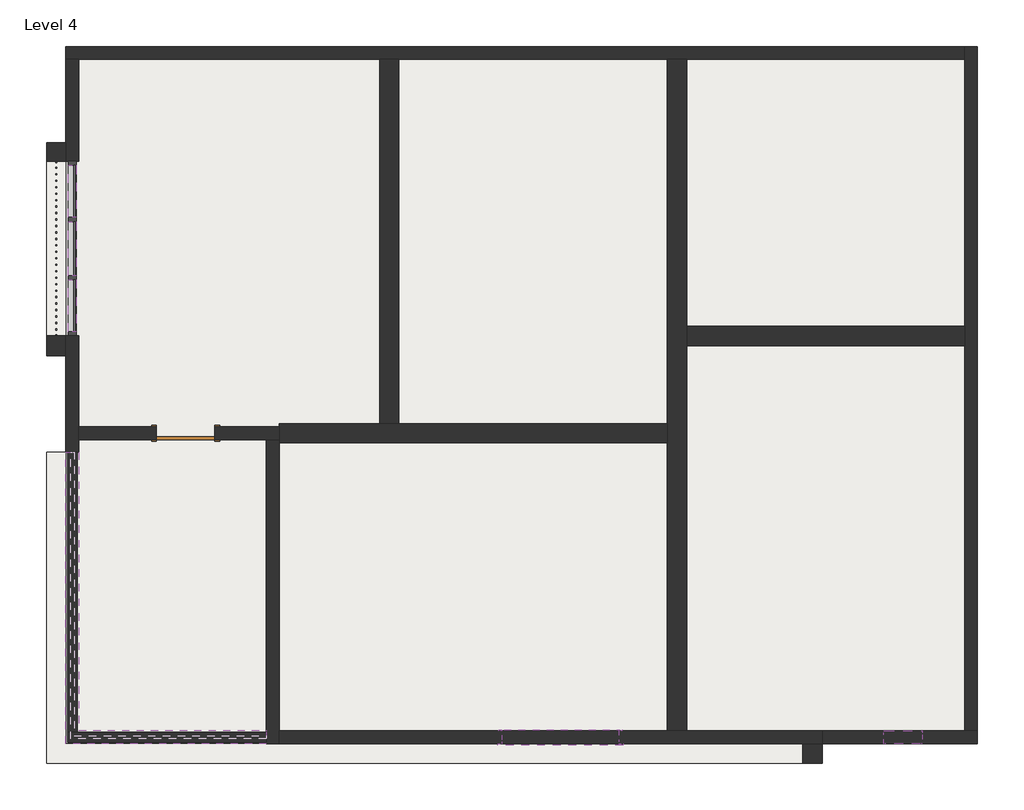
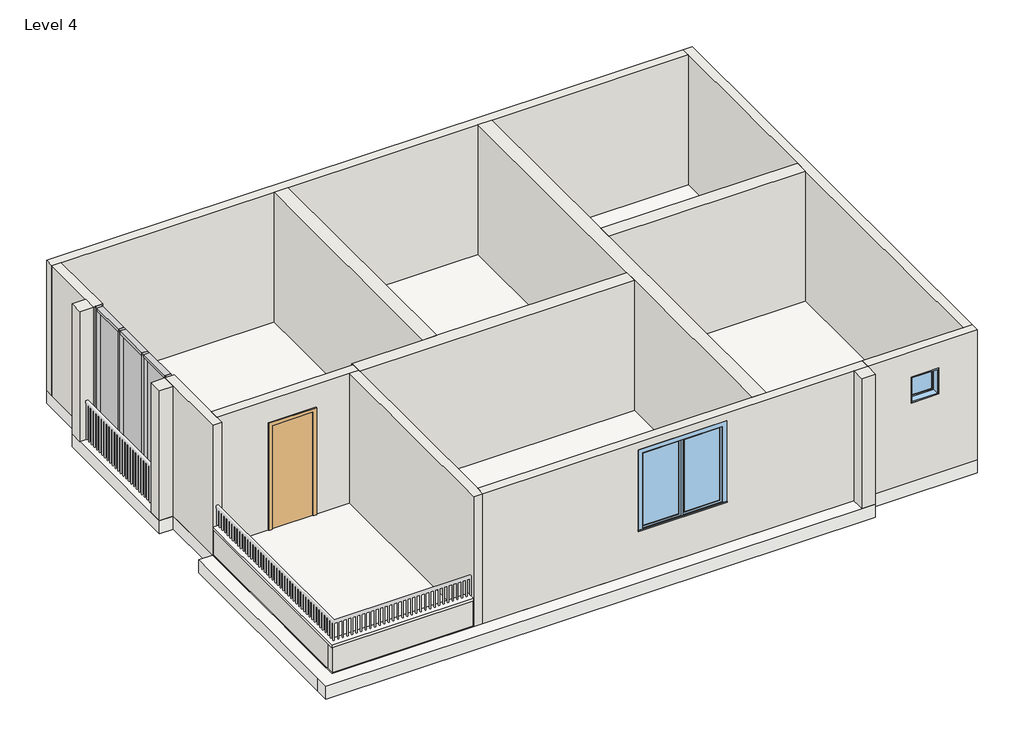
# One storey, part 1 of 2: 17 walls, 10 members, 3 plates, 3 slabs, 2 windows, 1 door.
"""IFC4 building model written with IfcOpenShell, lengths in millimetres."""

from ifc_helpers import new_model, si_unit, frame, origin, place, context, project, spatial, polyline, outline, extrude, faceted_brep, transform, mapped, element, save
from components import door_f936a269, member_eaba9652, member_3f395ae9, member_c17f1be2, member_d2e7e466, system_panel_glazed_52d31088, system_panel_glazed_f0722de2, window_97c6202a, window_6846e476

model = new_model("IFC4")

# Units and contexts
model_context = context("Model", 3, world=origin())
ifc_project = project(units=[si_unit("LENGTHUNIT", "METRE", prefix="MILLI")], contexts=[model_context])

# Site, building, storey
site = spatial("IfcSite", under=ifc_project)
building = spatial("IfcBuilding", under=site)
storey = spatial("IfcBuildingStorey", under=building, Name="Level 4", Elevation=9144.0)

# Door
placement = place(None, origin())
door_shape = door_f936a269(model_context)
element("IfcDoor", 1, ObjectType="Single-Flush : 36\" x 96\"", at=placement, inside=storey, context=model_context, shape_type="MappedRepresentation", body=[
    mapped(door_shape, transform((-16449.2169582, -4610.4617616, 10058.4), x_axis=(-1.0, 0.0, 0.0), y_axis=(0.0, -1.0, 0.0), z_axis=(0.0, 0.0, 1.0))),
])

# Members
member_shape = member_eaba9652(model_context)
element("IfcMember", 2, ObjectType="Rectangular Mullion : 2.5\" x 5\" rectangular", at=placement, inside=storey, context=model_context, shape_type="MappedRepresentation", body=[
    mapped(member_shape, transform((-18227.2169582, -1251.3117616, 10058.4), x_axis=(0.0, -1.0, 0.0), y_axis=(-1.0, 0.0, 0.0), z_axis=(0.0, 0.0, -1.0))),
])
element("IfcMember", 3, ObjectType="Rectangular Mullion : 2.5\" x 5\" rectangular", at=placement, inside=storey, context=model_context, shape_type="MappedRepresentation", body=[
    mapped(member_shape, transform((-18227.2169582, -2165.7117616, 10058.4), x_axis=(0.0, -1.0, 0.0), y_axis=(-1.0, 0.0, 0.0), z_axis=(0.0, 0.0, -1.0))),
])
member_2_shape = member_3f395ae9(model_context)
element("IfcMember", 4, ObjectType="Rectangular Mullion : 2.5\" x 5\" rectangular", at=placement, inside=storey, context=model_context, shape_type="MappedRepresentation", body=[
    mapped(member_2_shape, transform((-18227.2169582, -3080.1117616, 10058.4), x_axis=(0.0, -1.0, 0.0), y_axis=(-1.0, 0.0, 0.0), z_axis=(0.0, 0.0, -1.0))),
])
element("IfcMember", 5, ObjectType="Rectangular Mullion : 2.5\" x 5\" rectangular", at=placement, inside=storey, context=model_context, shape_type="MappedRepresentation", body=[
    mapped(member_2_shape, transform((-18227.2169582, -336.9117616, 13106.4), x_axis=(0.0, 1.0, 0.0), y_axis=(-1.0, 0.0, 0.0), z_axis=(0.0, 0.0, 1.0))),
])
member_3_shape = member_c17f1be2(model_context)
element("IfcMember", 6, ObjectType="Rectangular Mullion : 2.5\" x 5\" rectangular", at=placement, inside=storey, context=model_context, shape_type="MappedRepresentation", body=[
    mapped(member_3_shape, transform((-18227.2169582, -3016.6117616, 13106.4), x_axis=(0.0, 0.0, 1.0), y_axis=(-1.0, 0.0, 0.0), z_axis=(0.0, -1.0, 0.0))),
])
element("IfcMember", 7, ObjectType="Rectangular Mullion : 2.5\" x 5\" rectangular", at=placement, inside=storey, context=model_context, shape_type="MappedRepresentation", body=[
    mapped(member_3_shape, transform((-18227.2169582, -1219.5617616, 13106.4), x_axis=(0.0, 0.0, 1.0), y_axis=(-1.0, 0.0, 0.0), z_axis=(0.0, -1.0, 0.0))),
])
element("IfcMember", 8, ObjectType="Rectangular Mullion : 2.5\" x 5\" rectangular", at=placement, inside=storey, context=model_context, shape_type="MappedRepresentation", body=[
    mapped(member_3_shape, transform((-18227.2169582, -400.4117616, 10058.4), x_axis=(0.0, 0.0, -1.0), y_axis=(-1.0, 0.0, 0.0), z_axis=(0.0, 1.0, 0.0))),
])
element("IfcMember", 9, ObjectType="Rectangular Mullion : 2.5\" x 5\" rectangular", at=placement, inside=storey, context=model_context, shape_type="MappedRepresentation", body=[
    mapped(member_3_shape, transform((-18227.2169582, -2197.4617616, 10058.4), x_axis=(0.0, 0.0, -1.0), y_axis=(-1.0, 0.0, 0.0), z_axis=(0.0, 1.0, 0.0))),
])
member_4_shape = member_d2e7e466(model_context)
element("IfcMember", 10, ObjectType="Rectangular Mullion : 2.5\" x 5\" rectangular", at=placement, inside=storey, context=model_context, shape_type="MappedRepresentation", body=[
    mapped(member_4_shape, transform((-18227.2169582, -1283.0617616, 10058.4), x_axis=(0.0, 0.0, -1.0), y_axis=(-1.0, 0.0, 0.0), z_axis=(0.0, 1.0, 0.0))),
])
element("IfcMember", 11, ObjectType="Rectangular Mullion : 2.5\" x 5\" rectangular", at=placement, inside=storey, context=model_context, shape_type="MappedRepresentation", body=[
    mapped(member_4_shape, transform((-18227.2169582, -2133.9617616, 13106.4), x_axis=(0.0, 0.0, 1.0), y_axis=(-1.0, 0.0, 0.0), z_axis=(0.0, -1.0, 0.0))),
])

# Plates
system_panel_glazed_shape = system_panel_glazed_52d31088(model_context)
element("IfcPlate", 12, ObjectType="System Panel : Glazed", at=placement, inside=storey, context=model_context, shape_type="MappedRepresentation", body=[
    mapped(system_panel_glazed_shape, transform((-18227.2169582, -809.9867616, 10121.9), x_axis=(0.0, -1.0, 0.0), y_axis=(1.0, 0.0, 0.0), z_axis=(0.0, 0.0, 1.0))),
])
element("IfcPlate", 13, ObjectType="System Panel : Glazed", at=placement, inside=storey, context=model_context, shape_type="MappedRepresentation", body=[
    mapped(system_panel_glazed_shape, transform((-18227.2169582, -2607.0367616, 10121.9), x_axis=(0.0, -1.0, 0.0), y_axis=(1.0, 0.0, 0.0), z_axis=(0.0, 0.0, 1.0))),
])
system_panel_glazed_2_shape = system_panel_glazed_f0722de2(model_context)
element("IfcPlate", 14, ObjectType="System Panel : Glazed", at=placement, inside=storey, context=model_context, shape_type="MappedRepresentation", body=[
    mapped(system_panel_glazed_2_shape, transform((-18227.2169582, -1708.5117616, 10121.9), x_axis=(0.0, -1.0, 0.0), y_axis=(1.0, 0.0, 0.0), z_axis=(0.0, 0.0, 1.0))),
])

# Slabs
element("IfcSlab", 15, ObjectType="Generic - 12\"", at=placement, inside=storey, context=model_context, shape_type="SweptSolid", body=[
    extrude(outline(polyline([(-18633.6169582, -41.6299243), (-18328.8169582, -41.6299243), (-18328.8169582, -3394.4299243), (-18633.6169582, -3394.4299243), (-18633.6169582, -41.6299243)])), frame((0.0, 0.0, 9753.6), z_axis=(0.0, 0.0, 1.0), x_axis=(1.0, 0.0, 0.0)), (0.0, 0.0, 1.0), 304.8),
    extrude(outline(polyline([(-18633.6169582, -4908.9117616), (-18328.8169582, -4908.9117616), (-18328.8169582, -9487.2617616), (-6444.7919582, -9487.2617616), (-6444.7919582, -9792.0617616), (-18633.6169582, -9792.0617616), (-18633.6169582, -9487.2617616), (-18633.6169582, -4908.9117616)])), frame((0.0, 0.0, 9753.6), z_axis=(0.0, 0.0, 1.0), x_axis=(1.0, 0.0, 0.0)), (0.0, 0.0, 1.0), 304.8),
])
element("IfcSlab", 16, ObjectType="Generic - 12\" 2", at=placement, inside=storey, context=model_context, shape_type="SweptSolid", body=[
    extrude(outline(polyline([(-4006.3919582, 1466.4882384), (-4006.3919582, -9487.2617616), (-18328.8169582, -9487.2617616), (-18328.8169582, 1466.4882384), (-4006.3919582, 1466.4882384)])), frame((0.0, 0.0, 9753.6), z_axis=(0.0, 0.0, 1.0), x_axis=(1.0, 0.0, 0.0)), (0.0, 0.0, 1.0), 304.8),
])
element("IfcSlab", 17, ObjectType="Generic - 2\"", at=placement, inside=storey, context=model_context, shape_type="SweptSolid", body=[
    extrude(outline(polyline([(-15179.2169582, -9487.2617616), (-18328.8169582, -9487.2617616), (-18328.8169582, -4908.9117616), (-18125.6169582, -4908.9117616), (-18125.6169582, -9277.7117616), (-15179.2169582, -9277.7117616), (-15179.2169582, -9309.4617616), (-15179.2169582, -9487.2617616)])), frame((0.0, 0.0, 10668.0), z_axis=(0.0, 0.0, 1.0), x_axis=(1.0, 0.0, 0.0)), (0.0, 0.0, 1.0), 50.8),
])

# Walls
element("IfcWall", 18, ObjectType="Generic - 12\" white", at=placement, inside=storey, context=model_context, shape_type="SweptSolid", body=[
    extrude(outline(polyline([(-18633.6169582, -336.9117616), (-18633.6169582, -41.6299243), (-18328.8169582, -41.6299243), (-18328.8169582, -336.9117616), (-18633.6169582, -336.9117616)])), frame((0.0, 0.0, 10058.4), z_axis=(0.0, 0.0, 1.0), x_axis=(1.0, 0.0, 0.0)), (0.0, 0.0, 1.0), 3048.0),
])
element("IfcWall", 19, ObjectType="Generic - 12\" white", at=placement, inside=storey, context=model_context, shape_type="SweptSolid", body=[
    extrude(outline(polyline([(-18328.8169582, -3080.1117616), (-18328.8169582, -3394.4299243), (-18633.6169582, -3394.4299243), (-18633.6169582, -3080.1117616), (-18328.8169582, -3080.1117616)])), frame((0.0, 0.0, 10058.4), z_axis=(0.0, 0.0, 1.0), x_axis=(1.0, 0.0, 0.0)), (0.0, 0.0, 1.0), 3048.0),
])
element("IfcWall", 20, ObjectType="Generic - 12\" white", at=placement, inside=storey, context=model_context, shape_type="SweptSolid", body=[
    extrude(outline(polyline([(-6749.5919582, -9487.2617616), (-6444.7919582, -9487.2617616), (-6444.7919582, -9792.0617616), (-6749.5919582, -9792.0617616), (-6749.5919582, -9487.2617616)])), frame((0.0, 0.0, 10058.4), z_axis=(0.0, 0.0, 1.0), x_axis=(1.0, 0.0, 0.0)), (0.0, 0.0, 1.0), 3048.0),
])
element("IfcWall", 21, ObjectType="Generic - 12\" white", at=placement, inside=storey, context=model_context, shape_type="Brep", body=[
    faceted_brep([(-8575.2169582, -9284.0617616, 10058.4), (-8575.2169582, -3232.5117616, 10058.4), (-8575.2169582, -2927.7117616, 10058.4), (-8575.2169582, 1263.2882384, 10058.4), (-8575.2169582, 1263.2882384, 13106.4), (-8575.2169582, -2927.7117616, 13106.4), (-8575.2169582, -3232.5117616, 13106.4), (-8575.2169582, -9284.0617616, 13106.4), (-8880.0169582, -9284.0617616, 10058.4), (-8880.0169582, -9284.0617616, 13106.4), (-8880.0169582, -4762.8617616, 13106.4), (-8880.0169582, -4458.0617616, 13106.4), (-8880.0169582, 1263.2882384, 13106.4), (-8880.0169582, 1263.2882384, 10058.4), (-8880.0169582, -4458.0617616, 10058.4), (-8880.0169582, -4762.8617616, 10058.4)], [[[0, 1, 2, 3, 4, 5, 6, 7]], [[8, 9, 10, 11, 12, 13, 14, 15]], [[3, 2, 1, 0, 8, 15, 14, 13]], [[7, 6, 5, 4, 12, 11, 10, 9]], [[4, 3, 13, 12]], [[0, 7, 9, 8]]]),
])
element("IfcWall", 22, ObjectType="Generic - 12\" white", at=placement, inside=storey, context=model_context, shape_type="Brep", body=[
    faceted_brep([(-14976.0169582, -4762.8617616, 10058.4), (-8880.0169582, -4762.8617616, 10058.4), (-8880.0169582, -4762.8617616, 13106.4), (-14976.0169582, -4762.8617616, 13106.4), (-14976.0169582, -4458.0617616, 10058.4), (-14976.0169582, -4458.0617616, 13106.4), (-13401.2169582, -4458.0617616, 13106.4), (-13096.4169582, -4458.0617616, 13106.4), (-8880.0169582, -4458.0617616, 13106.4), (-8880.0169582, -4458.0617616, 10058.4), (-13096.4169582, -4458.0617616, 10058.4), (-13401.2169582, -4458.0617616, 10058.4), (-14976.0169582, -4712.0617616, 10058.4), (-14976.0169582, -4508.8617616, 10058.4), (-14976.0169582, -4508.8617616, 13106.4), (-14976.0169582, -4712.0617616, 13106.4)], [[[0, 1, 2, 3]], [[4, 5, 6, 7, 8, 9, 10, 11]], [[1, 0, 12, 13, 4, 11, 10, 9]], [[3, 2, 8, 7, 6, 5, 14, 15]], [[0, 3, 15, 14, 5, 4, 13, 12]], [[2, 1, 9, 8]]]),
])
element("IfcWall", 23, ObjectType="Generic - 12\" white", at=placement, inside=storey, context=model_context, shape_type="SweptSolid", body=[
    extrude(outline(polyline([(-13096.4169582, 1263.2882384), (-13096.4169582, -4458.0617616), (-13401.2169582, -4458.0617616), (-13401.2169582, 1263.2882384), (-13096.4169582, 1263.2882384)])), frame((0.0, 0.0, 10058.4), z_axis=(0.0, 0.0, 1.0), x_axis=(1.0, 0.0, 0.0)), (0.0, 0.0, 1.0), 3048.0),
])
element("IfcWall", 24, ObjectType="Generic - 12\" white", at=placement, inside=storey, context=model_context, shape_type="SweptSolid", body=[
    extrude(outline(polyline([(-4209.5919582, -3232.5117616), (-8575.2169582, -3232.5117616), (-8575.2169582, -2927.7117616), (-4209.5919582, -2927.7117616), (-4209.5919582, -3232.5117616)])), frame((0.0, 0.0, 10058.4), z_axis=(0.0, 0.0, 1.0), x_axis=(1.0, 0.0, 0.0)), (0.0, 0.0, 1.0), 3048.0),
])
element("IfcWall", 25, ObjectType="Generic - 6\"", at=placement, inside=storey, context=model_context, shape_type="Brep", body=[
    faceted_brep([(-15179.2169582, -9309.4617616, 10058.4), (-18151.0169582, -9309.4617616, 10058.4), (-18303.4169582, -9309.4617616, 10058.4), (-18303.4169582, -9309.4617616, 10668.0), (-18151.0169582, -9309.4617616, 10668.0), (-15179.2169582, -9309.4617616, 10668.0), (-15179.2169582, -9461.8617616, 10058.4), (-15179.2169582, -9461.8617616, 10668.0), (-18303.4169582, -9461.8617616, 10668.0), (-18303.4169582, -9461.8617616, 10058.4)], [[[0, 1, 2, 3, 4, 5]], [[6, 7, 8, 9]], [[2, 1, 0, 6, 9]], [[5, 4, 3, 8, 7]], [[0, 5, 7, 6]], [[3, 2, 9, 8]]]),
])
element("IfcWall", 26, ObjectType="Generic - 6\"", at=placement, inside=storey, context=model_context, shape_type="SweptSolid", body=[
    extrude(outline(polyline([(-18151.0169582, -4908.9117616), (-18151.0169582, -9309.4617616), (-18303.4169582, -9309.4617616), (-18303.4169582, -4908.9117616), (-18151.0169582, -4908.9117616)])), frame((0.0, 0.0, 10058.4), z_axis=(0.0, 0.0, 1.0), x_axis=(1.0, 0.0, 0.0)), (0.0, 0.0, 1.0), 609.6),
])
element("IfcWall", 27, ObjectType="Generic - 8\"", at=placement, inside=storey, context=model_context, shape_type="Brep", body=[
    faceted_brep([(-4006.3919582, -9284.0617616, 10058.4), (-4006.3919582, 1466.4882384, 10058.4), (-4006.3919582, 1466.4882384, 13106.4), (-4006.3919582, -9284.0617616, 13106.4), (-4209.5919582, -9284.0617616, 10058.4), (-4209.5919582, -9284.0617616, 13106.4), (-4209.5919582, -3232.5117616, 13106.4), (-4209.5919582, -2927.7117616, 13106.4), (-4209.5919582, 1263.2882384, 13106.4), (-4209.5919582, 1466.4882384, 13106.4), (-4209.5919582, 1466.4882384, 10058.4), (-4209.5919582, 1263.2882384, 10058.4), (-4209.5919582, -2927.7117616, 10058.4), (-4209.5919582, -3232.5117616, 10058.4)], [[[0, 1, 2, 3]], [[4, 5, 6, 7, 8, 9, 10, 11, 12, 13]], [[1, 0, 4, 13, 12, 11, 10]], [[3, 2, 9, 8, 7, 6, 5]], [[0, 3, 5, 4]], [[2, 1, 10, 9]]]),
])
element("IfcWall", 28, ObjectType="Generic - 8\"", at=placement, inside=storey, context=model_context, shape_type="Brep", body=[
    faceted_brep([(-4209.5919582, 1466.4882384, 10058.4), (-18328.8169582, 1466.4882384, 10058.4), (-18328.8169582, 1466.4882384, 13106.4), (-4209.5919582, 1466.4882384, 13106.4), (-4209.5919582, 1263.2882384, 10058.4), (-4209.5919582, 1263.2882384, 13106.4), (-8575.2169582, 1263.2882384, 13106.4), (-8880.0169582, 1263.2882384, 13106.4), (-13096.4169582, 1263.2882384, 13106.4), (-13401.2169582, 1263.2882384, 13106.4), (-18125.6169582, 1263.2882384, 13106.4), (-18328.8169582, 1263.2882384, 13106.4), (-18328.8169582, 1263.2882384, 10058.4), (-18125.6169582, 1263.2882384, 10058.4), (-13401.2169582, 1263.2882384, 10058.4), (-13096.4169582, 1263.2882384, 10058.4), (-8880.0169582, 1263.2882384, 10058.4), (-8575.2169582, 1263.2882384, 10058.4)], [[[0, 1, 2, 3]], [[4, 5, 6, 7, 8, 9, 10, 11, 12, 13, 14, 15, 16, 17]], [[1, 0, 4, 17, 16, 15, 14, 13, 12]], [[3, 2, 11, 10, 9, 8, 7, 6, 5]], [[0, 3, 5, 4]], [[2, 1, 12, 11]]]),
])
element("IfcWall", 29, ObjectType="Generic - 8\"", at=placement, inside=storey, context=model_context, shape_type="SweptSolid", body=[
    extrude(outline(polyline([(-18328.8169582, -336.9117616), (-18328.8169582, 1263.2882384), (-18125.6169582, 1263.2882384), (-18125.6169582, -336.9117616), (-18328.8169582, -336.9117616)])), frame((0.0, 0.0, 10058.4), z_axis=(0.0, 0.0, 1.0), x_axis=(1.0, 0.0, 0.0)), (0.0, 0.0, 1.0), 3048.0),
])
element("IfcWall", 30, ObjectType="Generic - 8\"", at=placement, inside=storey, context=model_context, shape_type="Brep", body=[
    faceted_brep([(-18328.8169582, -3080.1117616, 10058.4), (-18328.8169582, -4908.9117616, 10058.4), (-18328.8169582, -4908.9117616, 13106.4), (-18328.8169582, -3080.1117616, 13106.4), (-18125.6169582, -3080.1117616, 10058.4), (-18125.6169582, -3080.1117616, 13106.4), (-18125.6169582, -4508.8617616, 13106.4), (-18125.6169582, -4712.0617616, 13106.4), (-18125.6169582, -4908.9117616, 13106.4), (-18125.6169582, -4908.9117616, 10058.4), (-18125.6169582, -4712.0617616, 10058.4), (-18125.6169582, -4508.8617616, 10058.4), (-18151.0169582, -4908.9117616, 10058.4), (-18303.4169582, -4908.9117616, 10058.4)], [[[0, 1, 2, 3]], [[4, 5, 6, 7, 8, 9, 10, 11]], [[1, 0, 4, 11, 10, 9, 12, 13]], [[2, 1, 13, 12, 9, 8]], [[3, 2, 8, 7, 6, 5]], [[0, 3, 5, 4]]]),
])
element("IfcWall", 31, ObjectType="Generic - 8\" 2", at=placement, inside=storey, context=model_context, shape_type="Brep", body=[
    faceted_brep([(-4006.3919582, -9284.0617616, 10058.4), (-4209.5919582, -9284.0617616, 10058.4), (-6444.7919582, -9284.0617616, 10058.4), (-6444.7919582, -9284.0617616, 13106.4), (-4209.5919582, -9284.0617616, 13106.4), (-4006.3919582, -9284.0617616, 13106.4), (-4869.9919582, -9284.0617616, 12514.6087386), (-5479.5919582, -9284.0617616, 12514.6087386), (-5479.5919582, -9284.0617616, 11905.0087386), (-4869.9919582, -9284.0617616, 11905.0087386), (-4006.3919582, -9487.2617616, 10058.4), (-4006.3919582, -9487.2617616, 13106.4), (-6444.7919582, -9487.2617616, 13106.4), (-6444.7919582, -9487.2617616, 10058.4), (-4869.9919582, -9487.2617616, 12514.6087386), (-4869.9919582, -9487.2617616, 11905.0087386), (-5479.5919582, -9487.2617616, 11905.0087386), (-5479.5919582, -9487.2617616, 12514.6087386)], [[[0, 1, 2, 3, 4, 5], [6, 7, 8, 9]], [[10, 11, 12, 13], [14, 15, 16, 17]], [[2, 1, 0, 10, 13]], [[3, 2, 13, 12]], [[5, 4, 3, 12, 11]], [[0, 5, 11, 10]], [[15, 14, 6, 9]], [[16, 15, 9, 8]], [[17, 16, 8, 7]], [[14, 17, 7, 6]]]),
])
element("IfcWall", 32, ObjectType="Generic - 8\" 3", at=placement, inside=storey, context=model_context, shape_type="Brep", body=[
    faceted_brep([(-14976.0169582, -4712.0617616, 13106.4), (-15179.2169582, -4712.0617616, 13106.4), (-18125.6169582, -4712.0617616, 13106.4), (-18125.6169582, -4712.0617616, 10058.4), (-16906.4169582, -4712.0617616, 10058.4), (-16906.4169582, -4712.0617616, 12496.8), (-15992.0169582, -4712.0617616, 12496.8), (-15992.0169582, -4712.0617616, 10058.4), (-15179.2169582, -4712.0617616, 10058.4), (-14976.0169582, -4712.0617616, 10058.4), (-18125.6169582, -4508.8617616, 13106.4), (-14976.0169582, -4508.8617616, 13106.4), (-14976.0169582, -4508.8617616, 10058.4), (-15992.0169582, -4508.8617616, 10058.4), (-15992.0169582, -4508.8617616, 12496.8), (-16906.4169582, -4508.8617616, 12496.8), (-16906.4169582, -4508.8617616, 10058.4), (-18125.6169582, -4508.8617616, 10058.4)], [[[0, 1, 2, 3, 4, 5, 6, 7, 8, 9]], [[10, 11, 12, 13, 14, 15, 16, 17]], [[3, 17, 16, 4]], [[12, 9, 8, 7, 13]], [[2, 1, 0, 11, 10]], [[3, 2, 10, 17]], [[0, 9, 12, 11]], [[15, 5, 4, 16]], [[5, 15, 14, 6]], [[6, 14, 13, 7]]]),
])
element("IfcWall", 33, ObjectType="Generic - 8\" 3", at=placement, inside=storey, context=model_context, shape_type="Brep", body=[
    faceted_brep([(-15179.2169582, -4712.0617616, 10058.4), (-15179.2169582, -9309.4617616, 10058.4), (-15179.2169582, -9461.8617616, 10058.4), (-15179.2169582, -9487.2617616, 10058.4), (-15179.2169582, -9487.2617616, 13106.4), (-15179.2169582, -4712.0617616, 13106.4), (-14976.0169582, -4712.0617616, 10058.4), (-14976.0169582, -4712.0617616, 13106.4), (-14976.0169582, -4762.8617616, 13106.4), (-14976.0169582, -9284.0617616, 13106.4), (-14976.0169582, -9487.2617616, 13106.4), (-14976.0169582, -9487.2617616, 10058.4), (-14976.0169582, -9284.0617616, 10058.4), (-14976.0169582, -4762.8617616, 10058.4)], [[[0, 1, 2, 3, 4, 5]], [[6, 7, 8, 9, 10, 11, 12, 13]], [[3, 2, 1, 0, 6, 13, 12, 11]], [[5, 4, 10, 9, 8, 7]], [[0, 5, 7, 6]], [[3, 11, 10, 4]]]),
])
element("IfcWall", 34, ObjectType="Generic - 8\" 3", at=placement, inside=storey, context=model_context, shape_type="Brep", body=[
    faceted_brep([(-6444.7919582, -9284.0617616, 10058.4), (-8575.2169582, -9284.0617616, 10058.4), (-8880.0169582, -9284.0617616, 10058.4), (-14976.0169582, -9284.0617616, 10058.4), (-14976.0169582, -9284.0617616, 13106.4), (-8880.0169582, -9284.0617616, 13106.4), (-8575.2169582, -9284.0617616, 13106.4), (-6444.7919582, -9284.0617616, 13106.4), (-11470.8169582, -9284.0617616, 12856.6375963), (-11470.8169582, -9284.0617616, 11027.8375963), (-9642.0169582, -9284.0617616, 11027.8375963), (-9642.0169582, -9284.0617616, 12856.6375963), (-6444.7919582, -9487.2617616, 10058.4), (-6444.7919582, -9487.2617616, 13106.4), (-14976.0169582, -9487.2617616, 13106.4), (-14976.0169582, -9487.2617616, 10058.4), (-11470.8169582, -9487.2617616, 12856.6375963), (-9642.0169582, -9487.2617616, 12856.6375963), (-9642.0169582, -9487.2617616, 11027.8375963), (-11470.8169582, -9487.2617616, 11027.8375963)], [[[0, 1, 2, 3, 4, 5, 6, 7], [8, 9, 10, 11]], [[12, 13, 14, 15], [16, 17, 18, 19]], [[3, 2, 1, 0, 12, 15]], [[7, 6, 5, 4, 14, 13]], [[0, 7, 13, 12]], [[3, 15, 14, 4]], [[9, 8, 16, 19]], [[10, 9, 19, 18]], [[11, 10, 18, 17]], [[8, 11, 17, 16]]]),
])

# Windows
window_shape = window_97c6202a(model_context)
element("IfcWindow", 35, ObjectType="Casement Dbl with Trim.0001 : 72\" x 72\"", at=placement, inside=storey, context=model_context, shape_type="MappedRepresentation", body=[
    mapped(window_shape, transform((-10556.4169582, -9366.6117616, 10113.4375963), x_axis=(-1.0, 0.0, 0.0), y_axis=(0.0, -1.0, 0.0), z_axis=(0.0, 0.0, 1.0))),
])
window_2_shape = window_6846e476(model_context)
element("IfcWindow", 36, ObjectType="Fixed : 24\" x 24\"", at=placement, inside=storey, context=model_context, shape_type="MappedRepresentation", body=[
    mapped(window_2_shape, transform((-5136.6919582, -9385.6617616, 10990.6087386), x_axis=(1.0, 0.0, 0.0), y_axis=(0.0, 1.0, 0.0), z_axis=(0.0, 0.0, 1.0))),
])

save(model, "model.ifc")

# Revit data of these elements
# Type "Single-Flush : 36\" x 96\""
#   Type Mark = "1"
#   Construction Type Id = "MDOOR"
#   Assembly Code = "C1020"
#   Analytic Construction = "Metal"
#   Thickness = 0' - 2"
#   Heat Transfer Coefficient (U) = 0.651978 BTU/(h·ft²·°F)
#   Height = 8' - 0"
#   Trim Projection Ext = 0' - 1"
#   Trim Projection Int = 0' - 1"
#   Trim Width = 0' - 3"
#   Width = 3' - 0"
#   Define Thermal Properties by = 1
#   Door Material = Glass, Clear Glazing
#   Frame Material = Iron, Ductile
#   Visual Light Transmittance = 0
#   Solar Heat Gain Coefficient = 0
#   Function = (empty or 0)
#   Wall Closure = (empty or 0)
# Type "Rectangular Mullion : 2.5\" x 5\" rectangular"
#   built-in parameter 1007304 = 0.416667 (stored number, unit not read)
#   built-in parameter 1007301 = 0.104167 (stored number, unit not read)
#   built-in parameter 1007300 = 0.104167 (stored number, unit not read)
# Type "System Panel : Glazed"
#   Construction Type Id = "GSP4R"
#   Analytic Construction = "1/8 in Pilkington single glazing"
#   Visual Light Transmittance = 0.9
#   Solar Heat Gain Coefficient = 0.86
#   Heat Transfer Coefficient (U) = 1.18115 BTU/(h·ft²·°F)
# Type "Generic - 12\""
#   Assembly Code = "B1010"
#   Function = 0
#   Layers, outside or top first: 1' - 0" "Parking Stripe" (function 1)
# Type "Generic - 12\" 2"
#   Assembly Code = "B1010"
#   Function = 0
#   Layers, outside or top first: 1' - 0" "Parking Stripe" (function 1)
# Type "Generic - 2\""
#   Assembly Code = "B1010"
#   Function = 0
#   Layers, outside or top first: 0' - 2" "Parking Stripe" (function 1)
# Type "Generic - 12\" white"
#   Assembly Code = "B2010"
#   Layers, outside or top first: 1' - 0" "Parking Stripe" (function 1)
# Type "Generic - 6\""
#   Assembly Code = "B2010"
#   Layers, outside or top first: 0' - 6" "Concrete Masonry Units" (function 1)
# Type "Generic - 8\""
#   Assembly Code = "B2010"
#   Layers, outside or top first: 0' - 8" "Door - Frame" (function 1)
# Type "Generic - 8\" 2"
#   Assembly Code = "B2010"
#   Layers, outside or top first: 0' - 8" "Door - Frame" (function 1)
# Type "Generic - 8\" 3"
#   Assembly Code = "B2010"
#   Layers, outside or top first: 0' - 8" "EIFS, Exterior Insulation" (function 1)
# Type "Casement Dbl with Trim.0001 : 72\" x 72\""
#   Type Mark = "10"
#   Construction Type Id = "GSP4R"
#   Assembly Code = "B2020100"
#   Analytic Construction = "1/8 in Pilkington single glazing"
#   Visual Light Transmittance = 0.9
#   Solar Heat Gain Coefficient = 0.78
#   Heat Transfer Coefficient (U) = 0.6496 BTU/(h·ft²·°F)
#   Height = 6' - 0"
#   Default Sill Height = 3' - 0"
#   Trim Projection - Ext. = 0' - 0 1/2"
#   Trim Projection - Int. = 0' - 0 3/4"
#   Trim Width - Exterior = 0' - 3 1/2"
#   Trim Width - Interior = 0' - 3 1/2"
#   Width = 6' - 0"
#   Window Inset = 0' - 0 3/4"
#   Define Thermal Properties by = 1
#   Glass Pane Material = Glass
#   Sash Material = Iron, Ductile
#   Trim Exterior Material = Iron, Ductile
#   Trim Interior Material = Iron, Ductile
#   Wall Closure = (empty or 0)
# Type "Fixed : 24\" x 24\""
#   Type Mark = "3"
#   Construction Type Id = "GSP4R"
#   Assembly Code = "B2020100"
#   Analytic Construction = "1/8 in Pilkington single glazing"
#   Visual Light Transmittance = 0.9
#   Solar Heat Gain Coefficient = 0.78
#   Heat Transfer Coefficient (U) = 0.6496 BTU/(h·ft²·°F)
#   Height = 2' - 0"
#   Default Sill Height = 3' - 0"
#   Width = 2' - 0"
#   Window Inset = 0' - 0 3/4"
#   Define Thermal Properties by = 1
#   Glass Pane Material = Glass
#   Sash Material = Iron, Ductile
#   Wall Closure = (empty or 0)
# Element 1 (IfcDoor, "Single-Flush : 36\" x 96\"")
#   Phase Created = New Construction
#   Materials on its faces: "Iron, Ductile", "Glass, Clear Glazing"
# Elements 2, 3, 4, 5, 6, 7, 8, 9, 10, 11 (IfcMember, "Rectangular Mullion : 2.5\" x 5\" rectangular")
#   Phase Created = New Construction
#   Materials on its faces: "Iron, Ductile"
# Elements 12, 13, 14 (IfcPlate, "System Panel : Glazed")
#   Phase Created = New Construction
#   Materials on its faces: "Glass"
# Element 15 (IfcSlab, "Generic - 12\"")
#   built-in parameter 1001955 = 3.14159 (stored number, unit not read)
#   Height Offset From Level = 3' - 0"
#   Phase Created = New Construction
#   Materials on its faces: "Parking Stripe"
# Element 16 (IfcSlab, "Generic - 12\" 2")
#   Height Offset From Level = 3' - 0"
#   Phase Created = New Construction
#   Materials on its faces: "Parking Stripe"
# Element 17 (IfcSlab, "Generic - 2\"")
#   built-in parameter 1001955 = -1.5708 (stored number, unit not read)
#   Height Offset From Level = 5' - 2"
#   Phase Created = New Construction
#   Materials on its faces: "Parking Stripe"
# Elements 18, 19, 20, 21, 22, 23, 24 (IfcWall, "Generic - 12\" white")
#   built-in parameter 1001111 = 3' - 0"
#   Top Offset = 0' - 0"
#   Base Offset = 3' - 0"
#   Unconnected Height = 10' - 0"
#   wall height = 10' - 0"
#   Phase Created = New Construction
#   Base Constraint = Level 4
#   Materials on its faces: "Parking Stripe"
# Elements 25, 26 (IfcWall, "Generic - 6\"")
#   built-in parameter 1001111 = 3' - 0"
#   Top Offset = 0' - 0"
#   Base Offset = 3' - 0"
#   Unconnected Height = 2' - 0"
#   wall height = 2' - 0"
#   Phase Created = New Construction
#   Base Constraint = Level 4
#   Materials on its faces: "Concrete Masonry Units"
# Elements 27, 28, 29, 30 (IfcWall, "Generic - 8\"")
#   built-in parameter 1001111 = 3' - 0"
#   Top Offset = 0' - 0"
#   Base Offset = 3' - 0"
#   Unconnected Height = 10' - 0"
#   wall height = 10' - 0"
#   Phase Created = New Construction
#   Base Constraint = Level 4
#   Materials on its faces: "Door - Frame"
# Element 31 (IfcWall, "Generic - 8\" 2")
#   built-in parameter 1001111 = 3' - 0"
#   Top Offset = 0' - 0"
#   Base Offset = 3' - 0"
#   Unconnected Height = 10' - 0"
#   wall height = 10' - 0"
#   Phase Created = New Construction
#   Base Constraint = Level 4
#   Materials on its faces: "Door - Frame"
# Elements 32, 33, 34 (IfcWall, "Generic - 8\" 3")
#   built-in parameter 1001111 = 3' - 0"
#   Top Offset = 0' - 0"
#   Base Offset = 3' - 0"
#   Unconnected Height = 10' - 0"
#   wall height = 10' - 0"
#   Phase Created = New Construction
#   Base Constraint = Level 4
#   Materials on its faces: "EIFS, Exterior Insulation"
# Element 35 (IfcWindow, "Casement Dbl with Trim.0001 : 72\" x 72\"")
#   Mark = "6"
#   Phase Created = New Construction
#   Materials on its faces: "Iron, Ductile", "Glass"
# Element 36 (IfcWindow, "Fixed : 24\" x 24\"")
#   Mark = "5"
#   Phase Created = New Construction
#   Materials on its faces: "Iron, Ductile", "Glass"
# Materials
#   "Glass, Clear Glazing": class "Glass", colour RGB 0 128 192, transparency 0.75, Description = "Clear glazing", Cost = 0
#   "Iron, Ductile": class "Metal", colour RGB 0 0 0, transparency 0, Description = "Ductile cast iron", Cost = 0
#   "Parking Stripe": class "Paint", colour RGB 250 250 91, transparency 0, Cost = 0
#   "Concrete Masonry Units": class "Masonry", colour RGB 227 227 227, transparency 0, Description = "Concrete masonry units", Cost = 0
#   "Door - Frame": colour RGB 118 70 51, transparency 0, Cost = 0
#   "EIFS, Exterior Insulation": class "Generic", colour RGB 127 127 127, transparency 0, Description = "EIFS - Exterior Insulation", Cost = 0
#   "Glass": class "Glass", colour RGB 0 128 192, transparency 0.75, Description = "Soda Lime Glass", Cost = 0
